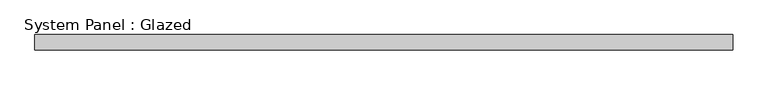
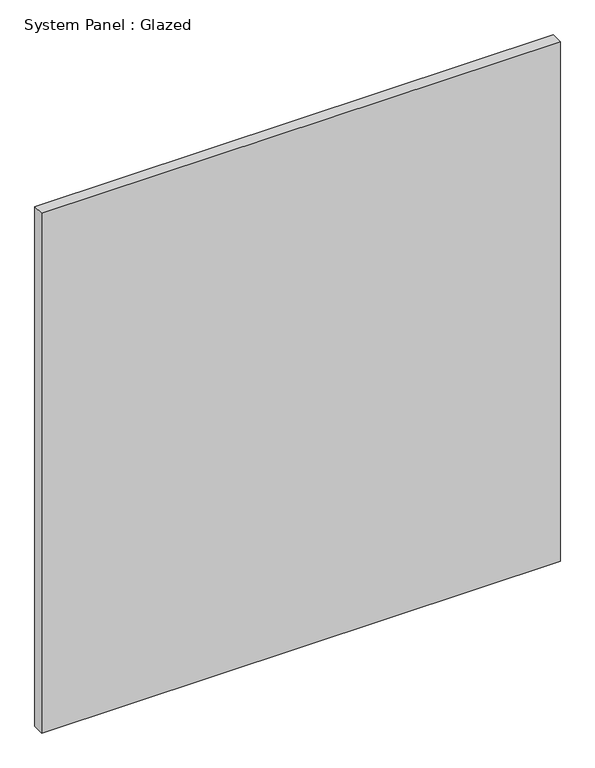
"""IFC4 building model written with IfcOpenShell, lengths in millimetres: plate geometry, System Panel : Glazed."""

from ifc_helpers import new_model, si_unit, origin, origin_with_axes, place, context, project, spatial, polyline, outline, extrude, source, transform, mapped, element, save


def system_panel_glazed_b869959d(model_context):
    return source(origin(), model_context, "Body", "SweptSolid", [
        extrude(outline(polyline([(572.42075, 19.05), (-572.42075, 19.05), (-572.42075, 44.45), (572.42075, 44.45), (572.42075, 19.05)])), origin_with_axes(), (0.0, 0.0, 1.0), 1211.961),
    ])


if __name__ == "__main__":
    model = new_model("IFC4")
    model_context = context("Model", 3, world=origin())
    ifc_project = project(units=[si_unit("LENGTHUNIT", "METRE", prefix="MILLI")], contexts=[model_context])
    site = spatial("IfcSite", under=ifc_project)
    building = spatial("IfcBuilding", under=site)
    placement = place(None, origin())
    system_panel_glazed_shape = system_panel_glazed_b869959d(model_context)
    element("IfcPlate", 1, ObjectType="System Panel : Glazed", at=placement, inside=building, context=model_context, shape_type="MappedRepresentation", body=[
        mapped(system_panel_glazed_shape, transform((0.0, 0.0, 0.0), x_axis=(1.0, 0.0, 0.0), y_axis=(0.0, 1.0, 0.0), z_axis=(0.0, 0.0, 1.0))),
    ])
    save(model, "model.ifc")

# Revit data of these elements
# Type "System Panel : Glazed"
#   Construction Type Id = "GSP4R"
#   Analytic Construction = "1/8 in Pilkington single glazing"
#   Visual Light Transmittance = 0.9
#   Solar Heat Gain Coefficient = 0.86
#   Heat Transfer Coefficient (U) = 1.18115 BTU/(h·ft²·°F)
#   Define Thermal Properties by = 1
# Element 1 (IfcPlate, "System Panel : Glazed")
#   Materials on its faces: "Glass"
# Materials
#   "Glass": class "Glass", colour RGB 0 128 192, transparency 0.75, Description = "Soda Lime Glass", Cost = 0
